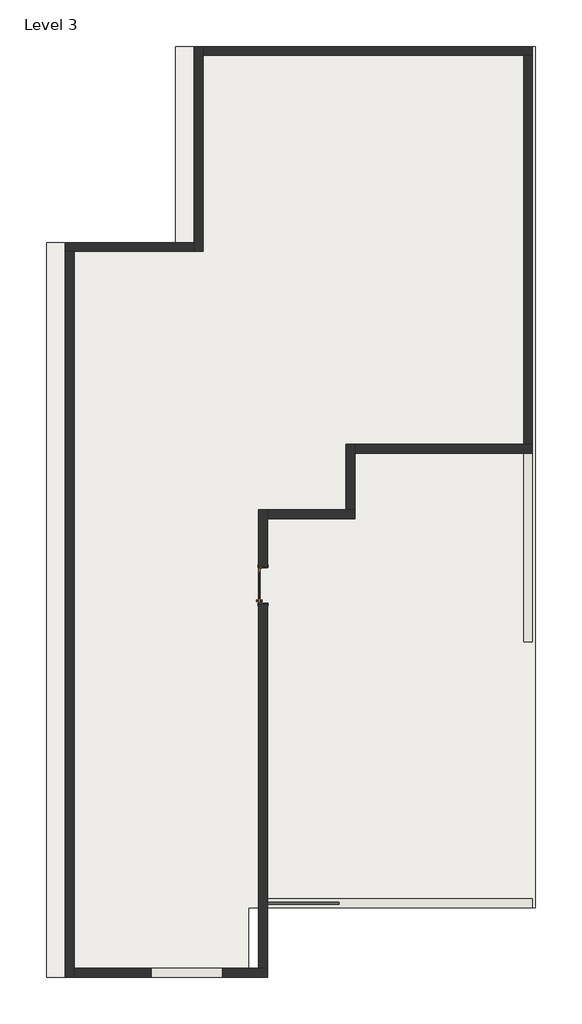
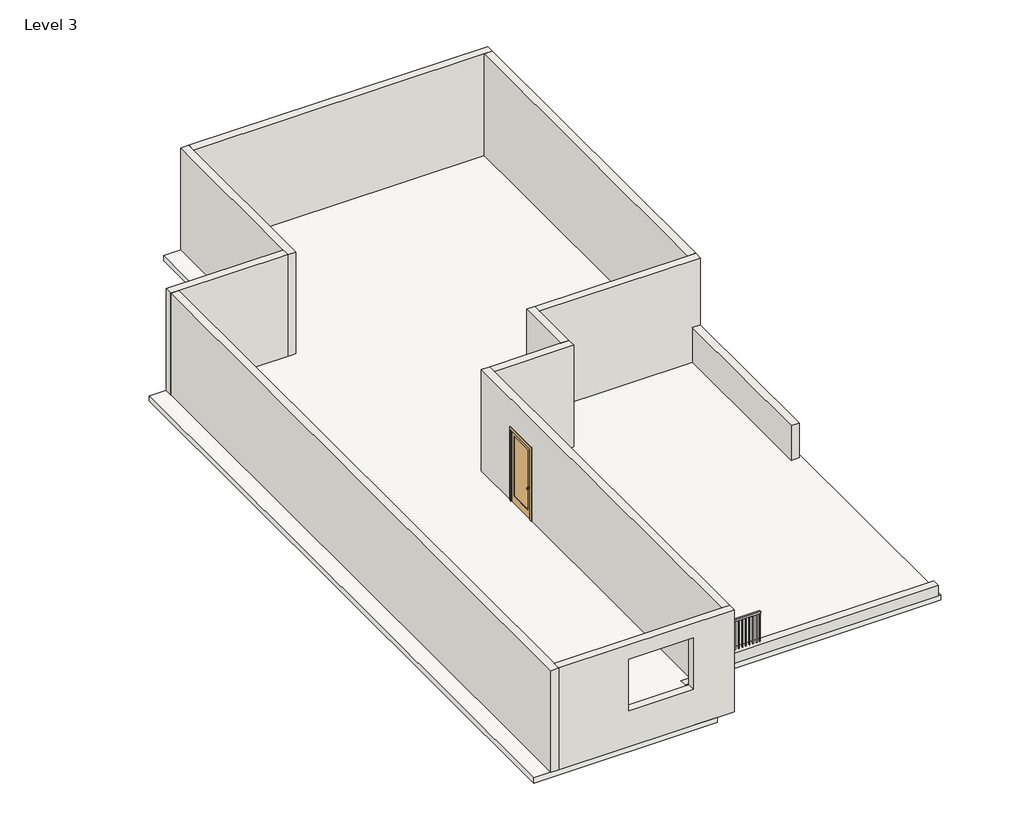
# One storey: 12 walls, 1 door, 1 railing, 1 slab.
"""IFC4 building model written with IfcOpenShell, lengths in millimetres."""

from ifc_helpers import new_model, si_unit, frame, origin, place, context, project, spatial, polyline, outline, extrude, faceted_brep, transform, mapped, element, save
from components import door_3b97b8e7

model = new_model("IFC4")

# Units and contexts
model_context = context("Model", 3, world=origin())
ifc_project = project(units=[si_unit("LENGTHUNIT", "METRE", prefix="MILLI")], contexts=[model_context])

# Site, building, storey
site = spatial("IfcSite", under=ifc_project)
building = spatial("IfcBuilding", under=site)
storey = spatial("IfcBuildingStorey", under=building, Name="Level 3", Elevation=3810.0)

# Door
placement = place(None, origin())
door_shape = door_3b97b8e7(model_context)
element("IfcDoor", 1, ObjectType="Door-Interior-Single-1_Panel-Wood : 36\" x 84\"", at=placement, inside=storey, context=model_context, shape_type="MappedRepresentation", body=[
    mapped(door_shape, transform((-8334.3925664, -3893.6444793, 3810.0), x_axis=(0.0, 1.0, 0.0), y_axis=(-1.0, 0.0, 0.0), z_axis=(0.0, 0.0, 1.0))),
])

# Railing
element("IfcRailing", 2, ObjectType="Handrail - Rectangular", at=placement, inside=storey, context=model_context, shape_type="SweptSolid", body=[
    extrude(outline(polyline([(-6385.0131952, -12021.6444793), (-6385.0131952, -12072.4444793), (-8216.9175664, -12072.4444793), (-8216.9175664, -12021.6444793), (-6385.0131952, -12021.6444793)])), frame((0.0, 0.0, 4978.4), z_axis=(0.0, 0.0, 1.0), x_axis=(1.0, 0.0, 0.0)), (0.0, 0.0, 1.0), 50.8),
    extrude(outline(polyline([(-8204.2881952, -12037.5194793), (-8204.2881952, -12056.5694793), (-8223.3381952, -12056.5694793), (-8223.3381952, -12037.5194793), (-8204.2881952, -12037.5194793)])), frame((0.0, 0.0, 4114.8), z_axis=(0.0, 0.0, 1.0), x_axis=(1.0, 0.0, 0.0)), (0.0, 0.0, 1.0), 863.6),
    extrude(outline(polyline([(-8102.6881952, -12037.5194793), (-8102.6881952, -12056.5694793), (-8121.7381952, -12056.5694793), (-8121.7381952, -12037.5194793), (-8102.6881952, -12037.5194793)])), frame((0.0, 0.0, 4114.8), z_axis=(0.0, 0.0, 1.0), x_axis=(1.0, 0.0, 0.0)), (0.0, 0.0, 1.0), 863.6),
    extrude(outline(polyline([(-8001.0881952, -12037.5194793), (-8001.0881952, -12056.5694793), (-8020.1381952, -12056.5694793), (-8020.1381952, -12037.5194793), (-8001.0881952, -12037.5194793)])), frame((0.0, 0.0, 4114.8), z_axis=(0.0, 0.0, 1.0), x_axis=(1.0, 0.0, 0.0)), (0.0, 0.0, 1.0), 863.6),
    extrude(outline(polyline([(-7899.4881952, -12037.5194793), (-7899.4881952, -12056.5694793), (-7918.5381952, -12056.5694793), (-7918.5381952, -12037.5194793), (-7899.4881952, -12037.5194793)])), frame((0.0, 0.0, 4114.8), z_axis=(0.0, 0.0, 1.0), x_axis=(1.0, 0.0, 0.0)), (0.0, 0.0, 1.0), 863.6),
    extrude(outline(polyline([(-7797.8881952, -12037.5194793), (-7797.8881952, -12056.5694793), (-7816.9381952, -12056.5694793), (-7816.9381952, -12037.5194793), (-7797.8881952, -12037.5194793)])), frame((0.0, 0.0, 4114.8), z_axis=(0.0, 0.0, 1.0), x_axis=(1.0, 0.0, 0.0)), (0.0, 0.0, 1.0), 863.6),
    extrude(outline(polyline([(-7696.2881952, -12037.5194793), (-7696.2881952, -12056.5694793), (-7715.3381952, -12056.5694793), (-7715.3381952, -12037.5194793), (-7696.2881952, -12037.5194793)])), frame((0.0, 0.0, 4114.8), z_axis=(0.0, 0.0, 1.0), x_axis=(1.0, 0.0, 0.0)), (0.0, 0.0, 1.0), 863.6),
    extrude(outline(polyline([(-7594.6881952, -12037.5194793), (-7594.6881952, -12056.5694793), (-7613.7381952, -12056.5694793), (-7613.7381952, -12037.5194793), (-7594.6881952, -12037.5194793)])), frame((0.0, 0.0, 4114.8), z_axis=(0.0, 0.0, 1.0), x_axis=(1.0, 0.0, 0.0)), (0.0, 0.0, 1.0), 863.6),
    extrude(outline(polyline([(-7493.0881952, -12037.5194793), (-7493.0881952, -12056.5694793), (-7512.1381952, -12056.5694793), (-7512.1381952, -12037.5194793), (-7493.0881952, -12037.5194793)])), frame((0.0, 0.0, 4114.8), z_axis=(0.0, 0.0, 1.0), x_axis=(1.0, 0.0, 0.0)), (0.0, 0.0, 1.0), 863.6),
    extrude(outline(polyline([(-7391.4881952, -12037.5194793), (-7391.4881952, -12056.5694793), (-7410.5381952, -12056.5694793), (-7410.5381952, -12037.5194793), (-7391.4881952, -12037.5194793)])), frame((0.0, 0.0, 4114.8), z_axis=(0.0, 0.0, 1.0), x_axis=(1.0, 0.0, 0.0)), (0.0, 0.0, 1.0), 863.6),
    extrude(outline(polyline([(-7289.8881952, -12037.5194793), (-7289.8881952, -12056.5694793), (-7308.9381952, -12056.5694793), (-7308.9381952, -12037.5194793), (-7289.8881952, -12037.5194793)])), frame((0.0, 0.0, 4114.8), z_axis=(0.0, 0.0, 1.0), x_axis=(1.0, 0.0, 0.0)), (0.0, 0.0, 1.0), 863.6),
    extrude(outline(polyline([(-7188.2881952, -12037.5194793), (-7188.2881952, -12056.5694793), (-7207.3381952, -12056.5694793), (-7207.3381952, -12037.5194793), (-7188.2881952, -12037.5194793)])), frame((0.0, 0.0, 4114.8), z_axis=(0.0, 0.0, 1.0), x_axis=(1.0, 0.0, 0.0)), (0.0, 0.0, 1.0), 863.6),
    extrude(outline(polyline([(-7086.6881952, -12037.5194793), (-7086.6881952, -12056.5694793), (-7105.7381952, -12056.5694793), (-7105.7381952, -12037.5194793), (-7086.6881952, -12037.5194793)])), frame((0.0, 0.0, 4114.8), z_axis=(0.0, 0.0, 1.0), x_axis=(1.0, 0.0, 0.0)), (0.0, 0.0, 1.0), 863.6),
    extrude(outline(polyline([(-6985.0881952, -12037.5194793), (-6985.0881952, -12056.5694793), (-7004.1381952, -12056.5694793), (-7004.1381952, -12037.5194793), (-6985.0881952, -12037.5194793)])), frame((0.0, 0.0, 4114.8), z_axis=(0.0, 0.0, 1.0), x_axis=(1.0, 0.0, 0.0)), (0.0, 0.0, 1.0), 863.6),
    extrude(outline(polyline([(-6883.4881952, -12037.5194793), (-6883.4881952, -12056.5694793), (-6902.5381952, -12056.5694793), (-6902.5381952, -12037.5194793), (-6883.4881952, -12037.5194793)])), frame((0.0, 0.0, 4114.8), z_axis=(0.0, 0.0, 1.0), x_axis=(1.0, 0.0, 0.0)), (0.0, 0.0, 1.0), 863.6),
    extrude(outline(polyline([(-6781.8881952, -12037.5194793), (-6781.8881952, -12056.5694793), (-6800.9381952, -12056.5694793), (-6800.9381952, -12037.5194793), (-6781.8881952, -12037.5194793)])), frame((0.0, 0.0, 4114.8), z_axis=(0.0, 0.0, 1.0), x_axis=(1.0, 0.0, 0.0)), (0.0, 0.0, 1.0), 863.6),
    extrude(outline(polyline([(-6680.2881952, -12037.5194793), (-6680.2881952, -12056.5694793), (-6699.3381952, -12056.5694793), (-6699.3381952, -12037.5194793), (-6680.2881952, -12037.5194793)])), frame((0.0, 0.0, 4114.8), z_axis=(0.0, 0.0, 1.0), x_axis=(1.0, 0.0, 0.0)), (0.0, 0.0, 1.0), 863.6),
    extrude(outline(polyline([(-6578.6881952, -12037.5194793), (-6578.6881952, -12056.5694793), (-6597.7381952, -12056.5694793), (-6597.7381952, -12037.5194793), (-6578.6881952, -12037.5194793)])), frame((0.0, 0.0, 4114.8), z_axis=(0.0, 0.0, 1.0), x_axis=(1.0, 0.0, 0.0)), (0.0, 0.0, 1.0), 863.6),
    extrude(outline(polyline([(-6477.0881952, -12037.5194793), (-6477.0881952, -12056.5694793), (-6496.1381952, -12056.5694793), (-6496.1381952, -12037.5194793), (-6477.0881952, -12037.5194793)])), frame((0.0, 0.0, 4114.8), z_axis=(0.0, 0.0, 1.0), x_axis=(1.0, 0.0, 0.0)), (0.0, 0.0, 1.0), 863.6),
    extrude(outline(polyline([(-8197.8675664, -12037.5194793), (-8197.8675664, -12056.5694793), (-8216.9175664, -12056.5694793), (-8216.9175664, -12037.5194793), (-8197.8675664, -12037.5194793)])), frame((0.0, 0.0, 4114.8), z_axis=(0.0, 0.0, 1.0), x_axis=(1.0, 0.0, 0.0)), (0.0, 0.0, 1.0), 863.6),
    extrude(outline(polyline([(-6385.0131952, -12037.5194793), (-6385.0131952, -12056.5694793), (-6404.0631952, -12056.5694793), (-6404.0631952, -12037.5194793), (-6385.0131952, -12037.5194793)])), frame((0.0, 0.0, 4114.8), z_axis=(0.0, 0.0, 1.0), x_axis=(1.0, 0.0, 0.0)), (0.0, 0.0, 1.0), 863.6),
])

# Slab
element("IfcSlab", 3, ObjectType="ground floor 6\"", at=placement, inside=storey, context=model_context, shape_type="SweptSolid", body=[
    extrude(outline(polyline([(-10580.3403048, 9936.6555207), (-1334.7403048, 9936.6555207), (-1334.7403048, -12161.3444793), (-8699.5175664, -12161.3444793), (-8699.5175664, -13952.0444793), (-13893.6629606, -13952.0444793), (-13893.6629606, 4907.4555207), (-10580.3403048, 4907.4555207), (-10580.3403048, 9936.6555207)])), frame((0.0, 0.0, 3657.6), z_axis=(0.0, 0.0, 1.0), x_axis=(1.0, 0.0, 0.0)), (0.0, 0.0, 1.0), 152.4),
])

# Walls
element("IfcWall", 4, ObjectType="9\" wall", at=placement, inside=storey, context=model_context, shape_type="Brep", body=[
    faceted_brep([(-10097.7403048, 9936.6555207, 3810.0), (-10097.7403048, 4907.4555207, 3810.0), (-10097.7403048, 4678.8555207, 3810.0), (-10097.7403048, 4678.8555207, 6858.0), (-10097.7403048, 4907.4555207, 6858.0), (-10097.7403048, 9936.6555207, 6858.0), (-9869.1403048, 9936.6555207, 3810.0), (-9869.1403048, 9936.6555207, 6858.0), (-9869.1403048, 9708.0555207, 6858.0), (-9869.1403048, 4678.8555207, 6858.0), (-9869.1403048, 4678.8555207, 3810.0), (-9869.1403048, 9708.0555207, 3810.0)], [[[0, 1, 2, 3, 4, 5]], [[6, 7, 8, 9, 10, 11]], [[2, 1, 0, 6, 11, 10]], [[5, 4, 3, 9, 8, 7]], [[3, 2, 10, 9]], [[0, 5, 7, 6]]]),
])
element("IfcWall", 5, ObjectType="9\" wall", at=placement, inside=storey, context=model_context, shape_type="Brep", body=[
    faceted_brep([(-1410.9403048, 9936.6555207, 3810.0), (-9869.1403048, 9936.6555207, 3810.0), (-9869.1403048, 9936.6555207, 6858.0), (-1410.9403048, 9936.6555207, 6858.0), (-1410.9403048, 9708.0555207, 3810.0), (-1410.9403048, 9708.0555207, 6858.0), (-1639.5403048, 9708.0555207, 6858.0), (-9869.1403048, 9708.0555207, 6858.0), (-9869.1403048, 9708.0555207, 3810.0), (-1639.5403048, 9708.0555207, 3810.0)], [[[0, 1, 2, 3]], [[4, 5, 6, 7, 8, 9]], [[1, 0, 4, 9, 8]], [[3, 2, 7, 6, 5]], [[2, 1, 8, 7]], [[0, 3, 5, 4]]]),
])
element("IfcWall", 6, ObjectType="9\" wall", at=placement, inside=storey, context=model_context, shape_type="Brep", body=[
    faceted_brep([(-13411.0629606, 4678.8555207, 3810.0), (-13182.4629606, 4678.8555207, 3810.0), (-10097.7403048, 4678.8555207, 3810.0), (-10097.7403048, 4678.8555207, 6858.0), (-13182.4629606, 4678.8555207, 6858.0), (-13411.0629606, 4678.8555207, 6858.0), (-13411.0629606, 4907.4555207, 3810.0), (-13411.0629606, 4907.4555207, 6858.0), (-10097.7403048, 4907.4555207, 6858.0), (-10097.7403048, 4907.4555207, 3810.0)], [[[0, 1, 2, 3, 4, 5]], [[6, 7, 8, 9]], [[2, 1, 0, 6, 9]], [[5, 4, 3, 8, 7]], [[3, 2, 9, 8]], [[0, 5, 7, 6]]]),
])
element("IfcWall", 7, ObjectType="9\" wall", at=placement, inside=storey, context=model_context, shape_type="Brep", body=[
    faceted_brep([(-8216.9175664, -13723.4444793, 3810.0), (-8445.5175664, -13723.4444793, 3810.0), (-13182.4629606, -13723.4444793, 3810.0), (-13182.4629606, -13723.4444793, 6858.0), (-8445.5175664, -13723.4444793, 6858.0), (-8216.9175664, -13723.4444793, 6858.0), (-9372.6175664, -13723.4444793, 4876.8), (-9372.6175664, -13723.4444793, 6426.2), (-11201.4175664, -13723.4444793, 6426.2), (-11201.4175664, -13723.4444793, 4876.8), (-13182.4629606, -13952.0444793, 3810.0), (-8216.9175664, -13952.0444793, 3810.0), (-8216.9175664, -13952.0444793, 6858.0), (-13182.4629606, -13952.0444793, 6858.0), (-9372.6175664, -13952.0444793, 6426.2), (-9372.6175664, -13952.0444793, 4876.8), (-11201.4175664, -13952.0444793, 4876.8), (-11201.4175664, -13952.0444793, 6426.2)], [[[0, 1, 2, 3, 4, 5], [6, 7, 8, 9]], [[10, 11, 12, 13], [14, 15, 16, 17]], [[2, 1, 0, 11, 10]], [[5, 4, 3, 13, 12]], [[0, 5, 12, 11]], [[3, 2, 10, 13]], [[6, 15, 14, 7]], [[7, 14, 17, 8]], [[8, 17, 16, 9]], [[15, 6, 9, 16]]]),
])
element("IfcWall", 8, ObjectType="9\" wall", at=placement, inside=storey, context=model_context, shape_type="Brep", body=[
    faceted_brep([(-8445.5175664, -13723.4444793, 6858.0), (-8445.5175664, -1950.5444793, 6858.0), (-8445.5175664, -1950.5444793, 3810.0), (-8445.5175664, -3411.0444793, 3810.0), (-8445.5175664, -3411.0444793, 5969.0), (-8445.5175664, -4376.2444793, 5969.0), (-8445.5175664, -4376.2444793, 3810.0), (-8445.5175664, -13723.4444793, 3810.0), (-8216.9175664, -1950.5444793, 6858.0), (-8216.9175664, -2179.1444793, 6858.0), (-8216.9175664, -13723.4444793, 6858.0), (-8216.9175664, -13723.4444793, 3810.0), (-8216.9175664, -12161.3444793, 3810.0), (-8216.9175664, -11932.7444793, 3810.0), (-8216.9175664, -4376.2444793, 3810.0), (-8216.9175664, -4376.2444793, 5969.0), (-8216.9175664, -3411.0444793, 5969.0), (-8216.9175664, -3411.0444793, 3810.0), (-8216.9175664, -2179.1444793, 3810.0), (-8216.9175664, -1950.5444793, 3810.0)], [[[0, 1, 2, 3, 4, 5, 6, 7]], [[8, 9, 10, 11, 12, 13, 14, 15, 16, 17, 18, 19]], [[11, 7, 6, 14, 13, 12]], [[2, 19, 18, 17, 3]], [[1, 0, 10, 9, 8]], [[0, 7, 11, 10]], [[2, 1, 8, 19]], [[16, 4, 3, 17]], [[4, 16, 15, 5]], [[5, 15, 14, 6]]]),
])
element("IfcWall", 9, ObjectType="9\" wall", at=placement, inside=storey, context=model_context, shape_type="SweptSolid", body=[
    extrude(outline(polyline([(-8216.9175664, -11932.7444793), (-1410.9403048, -11932.7444793), (-1410.9403048, -12161.3444793), (-8216.9175664, -12161.3444793), (-8216.9175664, -11932.7444793)])), frame((0.0, 0.0, 3810.0), z_axis=(0.0, 0.0, 1.0), x_axis=(1.0, 0.0, 0.0)), (0.0, 0.0, 1.0), 304.8),
])
element("IfcWall", 10, ObjectType="9\" wall", at=placement, inside=storey, context=model_context, shape_type="Brep", body=[
    faceted_brep([(-13182.4629606, -13954.5978416, 3810.0), (-13182.4629606, -13952.0444793, 3810.0), (-13182.4629606, -13723.4444793, 3810.0), (-13182.4629606, 4678.8555207, 3810.0), (-13182.4629606, 4678.8555207, 6858.0), (-13182.4629606, -13723.4444793, 6858.0), (-13182.4629606, -13952.0444793, 6858.0), (-13182.4629606, -13954.5978416, 6858.0), (-13411.0629606, -13954.5978416, 3810.0), (-13411.0629606, -13954.5978416, 6858.0), (-13411.0629606, 4678.8555207, 6858.0), (-13411.0629606, 4678.8555207, 3810.0)], [[[0, 1, 2, 3, 4, 5, 6, 7]], [[8, 9, 10, 11]], [[3, 2, 1, 0, 8, 11]], [[7, 6, 5, 4, 10, 9]], [[0, 7, 9, 8]], [[4, 3, 11, 10]]]),
])
element("IfcWall", 11, ObjectType="9\" wall", at=placement, inside=storey, context=model_context, shape_type="Brep", body=[
    faceted_brep([(-8216.9175664, -2179.1444793, 3810.0), (-5969.0175664, -2179.1444793, 3810.0), (-5969.0175664, -2179.1444793, 6858.0), (-8216.9175664, -2179.1444793, 6858.0), (-8216.9175664, -1950.5444793, 3810.0), (-8216.9175664, -1950.5444793, 6858.0), (-6197.6175664, -1950.5444793, 6858.0), (-5969.0175664, -1950.5444793, 6858.0), (-5969.0175664, -1950.5444793, 3810.0), (-6197.6175664, -1950.5444793, 3810.0)], [[[0, 1, 2, 3]], [[4, 5, 6, 7, 8, 9]], [[1, 0, 4, 9, 8]], [[3, 2, 7, 6, 5]], [[0, 3, 5, 4]], [[2, 1, 8, 7]]]),
])
element("IfcWall", 12, ObjectType="9\" wall", at=placement, inside=storey, context=model_context, shape_type="Brep", body=[
    faceted_brep([(-5969.0175664, -1950.5444793, 3810.0), (-5969.0175664, -502.7444793, 3810.0), (-5969.0175664, -274.1444793, 3810.0), (-5969.0175664, -274.1444793, 6858.0), (-5969.0175664, -502.7444793, 6858.0), (-5969.0175664, -1950.5444793, 6858.0), (-6197.6175664, -1950.5444793, 3810.0), (-6197.6175664, -1950.5444793, 6858.0), (-6197.6175664, -274.1444793, 6858.0), (-6197.6175664, -274.1444793, 3810.0)], [[[0, 1, 2, 3, 4, 5]], [[6, 7, 8, 9]], [[2, 1, 0, 6, 9]], [[5, 4, 3, 8, 7]], [[0, 5, 7, 6]], [[3, 2, 9, 8]]]),
])
element("IfcWall", 13, ObjectType="9\" wall", at=placement, inside=storey, context=model_context, shape_type="Brep", body=[
    faceted_brep([(-5969.0175664, -502.7444793, 3810.0), (-1639.5403048, -502.7444793, 3810.0), (-1410.9403048, -502.7444793, 3810.0), (-1410.9403048, -502.7444793, 4854.3755369), (-1410.9403048, -502.7444793, 6858.0), (-5969.0175664, -502.7444793, 6858.0), (-5969.0175664, -274.1444793, 3810.0), (-5969.0175664, -274.1444793, 6858.0), (-1639.5403048, -274.1444793, 6858.0), (-1410.9403048, -274.1444793, 6858.0), (-1410.9403048, -274.1444793, 3810.0), (-1639.5403048, -274.1444793, 3810.0)], [[[0, 1, 2, 3, 4, 5]], [[6, 7, 8, 9, 10, 11]], [[2, 1, 0, 6, 11, 10]], [[5, 4, 9, 8, 7]], [[0, 5, 7, 6]], [[2, 10, 9, 4, 3]]]),
])
element("IfcWall", 14, ObjectType="9\" wall", at=placement, inside=storey, context=model_context, shape_type="SweptSolid", body=[
    extrude(outline(polyline([(-1639.5403048, -274.1444793), (-1639.5403048, 9708.0555207), (-1410.9403048, 9708.0555207), (-1410.9403048, -274.1444793), (-1639.5403048, -274.1444793)])), frame((0.0, 0.0, 3810.0), z_axis=(0.0, 0.0, 1.0), x_axis=(1.0, 0.0, 0.0)), (0.0, 0.0, 1.0), 3048.0),
])
element("IfcWall", 15, ObjectType="9\" wall", at=placement, inside=storey, context=model_context, shape_type="Brep", body=[
    faceted_brep([(-1410.9403048, -5341.4444793, 3810.0), (-1410.9403048, -502.7444793, 3810.0), (-1410.9403048, -502.7444793, 4854.3755369), (-1410.9403048, -5341.4444793, 4854.3755369), (-1410.9403048, -5341.4444793, 4738.1107206), (-1639.5403048, -5341.4444793, 3810.0), (-1639.5403048, -5341.4444793, 4738.1107206), (-1639.5403048, -5341.4444793, 4854.3755369), (-1639.5403048, -502.7444793, 4854.3755369), (-1639.5403048, -502.7444793, 3810.0)], [[[0, 1, 2, 3, 4]], [[5, 6, 7, 8, 9]], [[1, 0, 5, 9]], [[3, 2, 8, 7]], [[0, 4, 3, 7, 6, 5]], [[2, 1, 9, 8]]]),
])

save(model, "model.ifc")

# Revit data of these elements
# Type "Door-Interior-Single-1_Panel-Wood : 36\" x 84\""
#   Type Mark = "8"
#   Assembly Code = "C1020300"
#   Analytic Construction = "Wooden"
#   Top Rail = 0' - 4 11/16"
#   Thickness = 0' - 1 3/8"
#   Thermal Resistance (R) = 2.5876 (h·ft²·°F)/BTU
#   Swing Angle [instance default] = 90.00°
#   Stiles = 0' - 4 3/4"
#   Rough Width = 3' - 2"
#   Rough Height = 7' - 1"
#   Height = 7' - 0"
#   Width = 3' - 0"
#   Heat Transfer Coefficient (U) = 0.3865 BTU/(h·ft²·°F)
#   Bottom Rail = 0' - 9 1/8"
#   Trim Material = Cherry
#   Panel Material = Cherry
#   Frame Material = Cherry
#   Door Handle Material = Aluminum
#   Visual Light Transmittance = 0
#   Solar Heat Gain Coefficient = 0
#   Wall Closure = (empty or 0)
#   Function = (empty or 0)
# Type "Handrail - Rectangular"
#   Assembly Code = "C2010400"
#   built-in parameter 1008612 = 0.0416667 (stored number, unit not read)
#   built-in parameter 1008611 = 0.0416667 (stored number, unit not read)
#   built-in parameter 1008609 = 0.333333 (stored number, unit not read)
#   built-in parameter 1008604 = 0.166667 (stored number, unit not read)
#   built-in parameter 1008603 = 0.166667 (stored number, unit not read)
#   Railing Height = 3' - 0"
#   built-in parameter 1008630 = 2
#   built-in parameter 1008610 = 2
#   built-in parameter 1008618 = Baluster - Square : 3/4"
# Type "ground floor 6\""
#   Assembly Code = "B1010"
#   Function = 0
# Type "9\" wall"
#   Assembly Code = "B2010"
# Element 1 (IfcDoor, "Door-Interior-Single-1_Panel-Wood : 36\" x 84\"")
#   Swing Angle = 90.00°
#   Phase Created = New Construction
#   Materials on its faces: "Cherry", "Aluminum"
# Element 2 (IfcRailing, "Handrail - Rectangular")
#   built-in parameter 1008621 = 1 (stored number, unit not read)
#   Phase Created = New Construction
#   Materials on its faces: "mullion"
# Element 3 (IfcSlab, "ground floor 6\"")
#   built-in parameter 1001955 = 3.14159 (stored number, unit not read)
#   Height Offset From Level = 0' - 0"
#   Phase Created = New Construction
# Elements 4, 5, 6, 7, 8, 10, 11, 12, 13, 14 (IfcWall, "9\" wall")
#   Top Offset = 0' - 0"
#   Base Offset = 0' - 0"
#   wall height = 10' - 0"
#   Phase Created = New Construction
#   Base Constraint = Level 3
#   Top Constraint = Level 4
# Element 9 (IfcWall, "9\" wall")
#   Top Offset = -9' - 0"
#   Base Offset = 0' - 0"
#   wall height = 1' - 0"
#   Phase Created = New Construction
#   Base Constraint = Level 3
#   Top Constraint = Level 4
# Element 15 (IfcWall, "9\" wall")
#   Top Offset = -6' - 6.88285"
#   Base Offset = 0' - 0"
#   wall height = 3' - 5.11715"
#   Phase Created = New Construction
#   Base Constraint = Level 3
#   Top Constraint = Level 4
# Materials
#   "Cherry": class "Wood", colour RGB 226 177 128, transparency 0, Description = "Prunus Serotina", Cost = 0
#   "Aluminum": class "Metal", colour RGB 247 247 247, transparency 0, Description = "Aluminum 6061", Cost = 0
#   "mullion": class "Generic", colour RGB 120 120 120, transparency 0, Cost = 0
